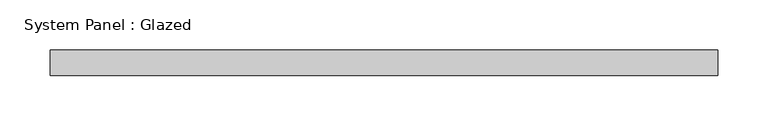
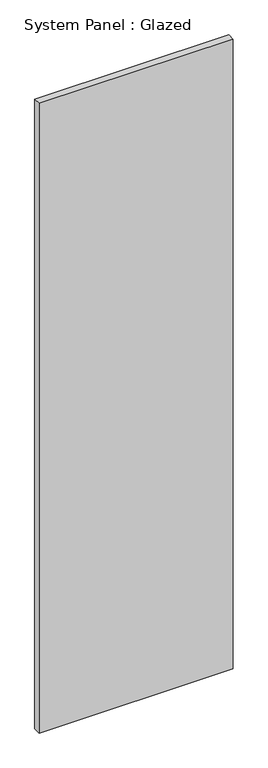
"""IFC4 building model written with IfcOpenShell, lengths in millimetres: plate geometry, System Panel : Glazed."""

from ifc_helpers import new_model, si_unit, origin, origin_with_axes, place, context, project, spatial, polyline, outline, extrude, source, transform, mapped, element, save


def system_panel_glazed_4d630f51(model_context):
    return source(origin(), model_context, "Body", "SweptSolid", [
        extrude(outline(polyline([(333.375, 19.05), (-333.375, 19.05), (-333.375, 44.45), (333.375, 44.45), (333.375, 19.05)])), origin_with_axes(), (0.0, 0.0, 1.0), 2284.5809615),
    ])


if __name__ == "__main__":
    model = new_model("IFC4")
    model_context = context("Model", 3, world=origin())
    ifc_project = project(units=[si_unit("LENGTHUNIT", "METRE", prefix="MILLI")], contexts=[model_context])
    site = spatial("IfcSite", under=ifc_project)
    building = spatial("IfcBuilding", under=site)
    placement = place(None, origin())
    system_panel_glazed_shape = system_panel_glazed_4d630f51(model_context)
    element("IfcPlate", 1, ObjectType="System Panel : Glazed", at=placement, inside=building, context=model_context, shape_type="MappedRepresentation", body=[
        mapped(system_panel_glazed_shape, transform((0.0, 0.0, 0.0), x_axis=(1.0, 0.0, 0.0), y_axis=(0.0, 1.0, 0.0), z_axis=(0.0, 0.0, 1.0))),
    ])
    save(model, "model.ifc")

# Revit data of these elements
# Type "System Panel : Glazed"
#   Construction Type Id = "GSP4R"
#   Analytic Construction = "1/8 in Pilkington single glazing"
#   Visual Light Transmittance = 0.9
#   Solar Heat Gain Coefficient = 0.86
#   Heat Transfer Coefficient (U) = 1.18115 BTU/(h·ft²·°F)
#   Define Thermal Properties by = 1
# Element 1 (IfcPlate, "System Panel : Glazed")
#   Materials on its faces: "Glass"
# Materials
#   "Glass": class "Glass", colour RGB 0 128 192, transparency 0.75, Description = "Soda Lime Glass", Cost = 0
